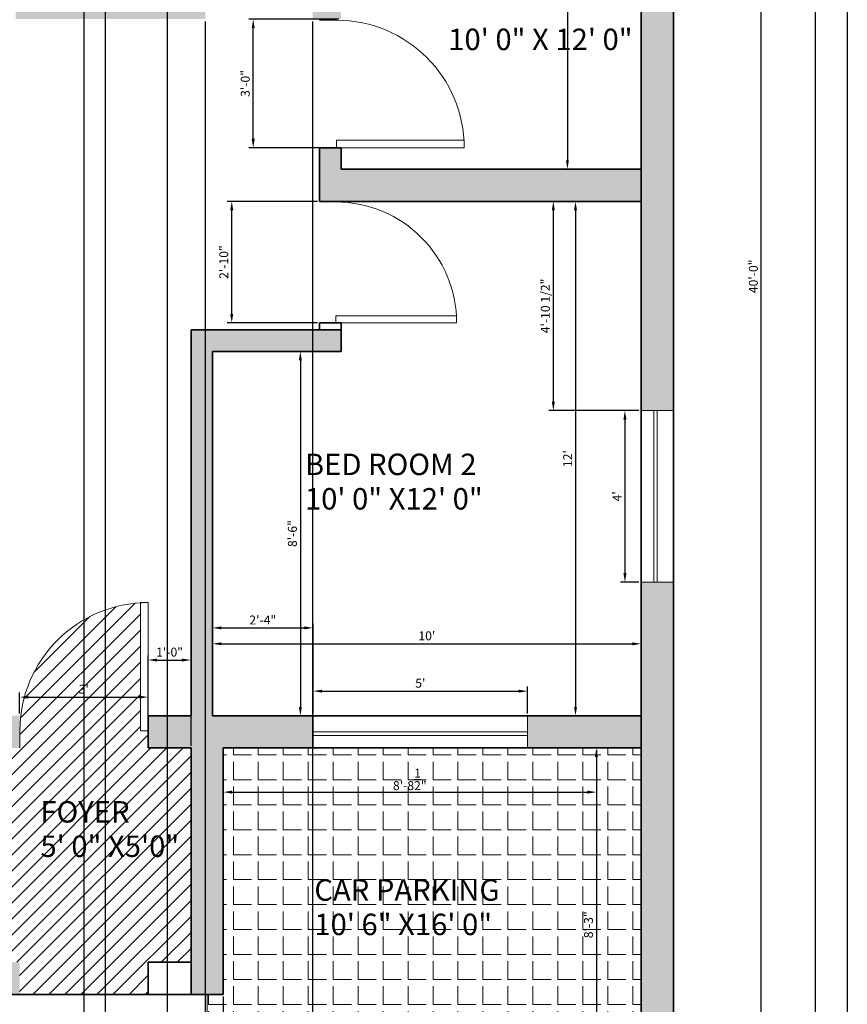
# Model space of a CAD drawing. Units: inches. Extents: x 2998 to 3448, y 1620 to 2377.
# Tile 3 of 5: x 3216 to 3448, y 1879 to 2155. Entities that reach past the tile are written whole.
import ezdxf

# ---------------------------------------------------------------- set-up
doc = ezdxf.new("R2010")
doc.units = ezdxf.units.IN
doc.layers.get('Defpoints').update_dxf_attribs({"color": 110})
for name, color, linetype, lineweight in [('A-ANNO-DIMS', 2, 'Continuous', 18), ('A-ANNO-TTLB', 7, 'Continuous', 25), ('A-AREA-IDEN', 130, 'Continuous', 18), ('A-DOOR', 3, 'Continuous', 18), ('A-FLOR-PATT', 18, 'Continuous', 13), ('A-GLAZ', 4, 'Continuous', 18), ('A-WALL-PATT', 18, 'Continuous', 13), ('C-PROP', 7, 'Continuous', 35), ('L-HRDS', 8, 'Continuous', 18), ('L-HRDS-PATT', 175, 'Continuous', 13), ('WALL', 7, 'Continuous', 35)]:
    doc.layers.add(name, color=color, linetype=linetype, lineweight=lineweight)
doc.styles.get("Standard").update_dxf_attribs({"font": 'arial.ttf'})
doc.dimstyles.new('Copy of ISO-25', dxfattribs={"dimtxt": 2.5, "dimasz": 2.5, "dimexe": 1.25, "dimexo": 0.625, "dimtad": 1, "dimdec": 1, "dimlunit": 4, "dimtxsty": 'Standard', "dimcen": 2.5, "dimadec": 0, "dimazin": 0, "dimtfac": 1, "dimtdec": 1, "dimtmove": 0, "dimatfit": 3, "dimfxl": 1, "dimarcsym": 0})

# ---------------------------------------------------------------- blocks, each defined once
blk = doc.blocks.new('*U3')
for p, q in [((-750, 0), (-750, -100)), ((0, 0), (0, -100))]:
    blk.add_line(p, q)
blk.add_lwpolyline([(0, 0), (0, 750), (-43.75, 750), (-43.75, 0)], close=True)
blk.add_arc((0, 0), 750, 90, 180)
blk = doc.blocks.new('*D4')
at = {"layer": 'A-ANNO-DIMS', "color": 0, "lineweight": -2, "transparency": 16777216}
for p, q in [((3389.49, 1950.77), (3376.33, 1950.77)), ((3377.58, 1948.27), (3377.58, 1854.27)), ((3389.49, 1851.77), (3376.33, 1851.77))]:
    blk.add_line(p, q, dxfattribs=at)
at = {"layer": 'A-ANNO-DIMS', "color": 0, "transparency": 16777216}
for points in [[(3377.16, 1948.27), (3378, 1948.27), (3377.58, 1950.77)], [(3377.16, 1854.27), (3378, 1854.27), (3377.58, 1851.77)]]:
    blk.add_solid(points, dxfattribs=at)
at = {"layer": 'Defpoints', "color": 0, "transparency": 16777216}
for p in [(3390.12, 1950.77), (3377.58, 1851.77), (3390.12, 1851.77)]:
    blk.add_point(p, dxfattribs=at)
at = {"layer": 'A-ANNO-DIMS', "color": 0, "transparency": 16777216, "insert": (3375.68, 1901.27), "char_height": 2.5, "attachment_point": 5, "rotation": 90}
blk.add_mtext('8\'-3"', dxfattribs=at)
blk = doc.blocks.new('*D13')
at = {"layer": 'A-ANNO-DIMS', "color": 0, "lineweight": -2, "transparency": 16777216}
for p, q in [((3389.49, 2256.77), (3368.21, 2256.77)), ((3369.46, 2254.27), (3369.46, 2115.27)), ((3389.49, 2112.77), (3368.21, 2112.77))]:
    blk.add_line(p, q, dxfattribs=at)
at = {"layer": 'A-ANNO-DIMS', "color": 0, "transparency": 16777216}
for points in [[(3369.04, 2254.27), (3369.87, 2254.27), (3369.46, 2256.77)], [(3369.04, 2115.27), (3369.87, 2115.27), (3369.46, 2112.77)]]:
    blk.add_solid(points, dxfattribs=at)
at = {"layer": 'Defpoints', "color": 0, "transparency": 16777216}
for p in [(3390.12, 2256.77), (3369.46, 2112.77), (3390.12, 2112.77)]:
    blk.add_point(p, dxfattribs=at)
at = {"layer": 'A-ANNO-DIMS', "color": 0, "transparency": 16777216, "insert": (3367.58, 2184.77), "char_height": 2.5, "attachment_point": 5, "rotation": 90}
blk.add_mtext("12'", dxfattribs=at)
blk = doc.blocks.new('*D14')
at = {"layer": 'A-ANNO-DIMS', "color": 0, "lineweight": -2, "transparency": 16777216}
for p, q in [((3270.12, 1960.4), (3270.12, 1981.17)), ((3272.62, 1979.92), (3387.62, 1979.92)), ((3390.12, 1960.4), (3390.12, 1981.17))]:
    blk.add_line(p, q, dxfattribs=at)
at = {"layer": 'A-ANNO-DIMS', "color": 0, "transparency": 16777216}
for points in [[(3272.62, 1980.33), (3272.62, 1979.5), (3270.12, 1979.92)], [(3387.62, 1980.33), (3387.62, 1979.5), (3390.12, 1979.92)]]:
    blk.add_solid(points, dxfattribs=at)
at = {"layer": 'Defpoints', "color": 0, "transparency": 16777216}
for p in [(3390.12, 1979.92), (3270.12, 1959.77), (3390.12, 1959.77)]:
    blk.add_point(p, dxfattribs=at)
at = {"layer": 'A-ANNO-DIMS', "color": 0, "transparency": 16777216, "insert": (3330.12, 1981.82), "char_height": 2.5, "attachment_point": 5}
blk.add_mtext("10'", dxfattribs=at)
blk = doc.blocks.new('*D15')
at = {"layer": 'A-ANNO-DIMS', "color": 0, "lineweight": -2, "transparency": 16777216}
for p, q in [((3389.49, 2103.77), (3370.48, 2103.77)), ((3371.73, 2101.27), (3371.73, 1962.27)), ((3389.49, 1959.77), (3370.48, 1959.77))]:
    blk.add_line(p, q, dxfattribs=at)
at = {"layer": 'A-ANNO-DIMS', "color": 0, "transparency": 16777216}
for points in [[(3371.31, 2101.27), (3372.14, 2101.27), (3371.73, 2103.77)], [(3371.31, 1962.27), (3372.14, 1962.27), (3371.73, 1959.77)]]:
    blk.add_solid(points, dxfattribs=at)
at = {"layer": 'Defpoints', "color": 0, "transparency": 16777216}
for p in [(3390.12, 2103.77), (3371.73, 1959.77), (3390.12, 1959.77)]:
    blk.add_point(p, dxfattribs=at)
at = {"layer": 'A-ANNO-DIMS', "color": 0, "transparency": 16777216, "insert": (3369.85, 2031.77), "char_height": 2.5, "attachment_point": 5, "rotation": 90}
blk.add_mtext("12'", dxfattribs=at)
blk = doc.blocks.new('*D16')
at = {"layer": 'A-ANNO-DIMS', "color": 0, "lineweight": -2, "transparency": 16777216}
for p, q in [((3273.12, 1950.15), (3273.12, 1937.14)), ((3377.58, 1950.15), (3377.58, 1937.14)), ((3275.62, 1938.39), (3375.08, 1938.39))]:
    blk.add_line(p, q, dxfattribs=at)
at = {"layer": 'A-ANNO-DIMS', "color": 0, "transparency": 16777216}
for points in [[(3275.62, 1938.81), (3275.62, 1937.97), (3273.12, 1938.39)], [(3375.08, 1938.81), (3375.08, 1937.97), (3377.58, 1938.39)]]:
    blk.add_solid(points, dxfattribs=at)
at = {"layer": 'Defpoints', "color": 0, "transparency": 16777216}
for p in [(3273.12, 1950.77), (3377.58, 1950.77), (3377.58, 1938.39)]:
    blk.add_point(p, dxfattribs=at)
at = {"layer": 'A-ANNO-DIMS', "color": 0, "transparency": 16777216, "insert": (3325.35, 1941.96), "char_height": 2.5, "attachment_point": 5}
blk.add_mtext('8\'-8{\\H1x;\\S1/2;}"', dxfattribs=at)
blk = doc.blocks.new('*D20')
at = {"layer": 'A-ANNO-DIMS', "color": 0, "lineweight": -2, "transparency": 16777216}
for p, q in [((3216.12, 1960.4), (3216.12, 1966.24)), ((3252.12, 1960.4), (3252.12, 1966.24)), ((3218.62, 1964.99), (3249.62, 1964.99))]:
    blk.add_line(p, q, dxfattribs=at)
at = {"layer": 'A-ANNO-DIMS', "color": 0, "transparency": 16777216}
for points in [[(3218.62, 1965.4), (3218.62, 1964.57), (3216.12, 1964.99)], [(3249.62, 1965.4), (3249.62, 1964.57), (3252.12, 1964.99)]]:
    blk.add_solid(points, dxfattribs=at)
at = {"layer": 'Defpoints', "color": 0, "transparency": 16777216}
for p in [(3252.12, 1964.99), (3216.12, 1959.77), (3252.12, 1959.77)]:
    blk.add_point(p, dxfattribs=at)
at = {"layer": 'A-ANNO-DIMS', "color": 0, "transparency": 16777216, "insert": (3234.12, 1966.89), "char_height": 2.5, "attachment_point": 5}
blk.add_mtext("3'", dxfattribs=at)
blk = doc.blocks.new('*D21')
at = {"layer": 'A-ANNO-DIMS', "color": 0, "lineweight": -2, "transparency": 16777216}
for p, q in [((3298.3, 1960.4), (3298.3, 1967.92)), ((3358.3, 1960.4), (3358.3, 1967.92)), ((3300.8, 1966.67), (3355.8, 1966.67))]:
    blk.add_line(p, q, dxfattribs=at)
at = {"layer": 'A-ANNO-DIMS', "color": 0, "transparency": 16777216}
for points in [[(3300.8, 1967.08), (3300.8, 1966.25), (3298.3, 1966.67)], [(3355.8, 1967.08), (3355.8, 1966.25), (3358.3, 1966.67)]]:
    blk.add_solid(points, dxfattribs=at)
at = {"layer": 'Defpoints', "color": 0, "transparency": 16777216}
for p in [(3358.3, 1966.67), (3298.3, 1959.77), (3358.3, 1959.77)]:
    blk.add_point(p, dxfattribs=at)
at = {"layer": 'A-ANNO-DIMS', "color": 0, "transparency": 16777216, "insert": (3328.3, 1968.56), "char_height": 2.5, "attachment_point": 5}
blk.add_mtext("5'", dxfattribs=at)
blk = doc.blocks.new('*D22')
at = {"layer": 'A-ANNO-DIMS', "color": 0, "lineweight": -2, "transparency": 16777216}
for p, q in [((3389.49, 2045.2), (3384.3, 2045.2)), ((3385.55, 2042.7), (3385.55, 1999.7)), ((3389.49, 1997.2), (3384.3, 1997.2))]:
    blk.add_line(p, q, dxfattribs=at)
at = {"layer": 'A-ANNO-DIMS', "color": 0, "transparency": 16777216}
for points in [[(3385.13, 2042.7), (3385.97, 2042.7), (3385.55, 2045.2)], [(3385.13, 1999.7), (3385.97, 1999.7), (3385.55, 1997.2)]]:
    blk.add_solid(points, dxfattribs=at)
at = {"layer": 'Defpoints', "color": 0, "transparency": 16777216}
for p in [(3390.12, 2045.2), (3385.55, 1997.2), (3390.12, 1997.2)]:
    blk.add_point(p, dxfattribs=at)
at = {"layer": 'A-ANNO-DIMS', "color": 0, "transparency": 16777216, "insert": (3383.68, 2021.2), "char_height": 2.5, "attachment_point": 5, "rotation": 90}
blk.add_mtext("4'", dxfattribs=at)
blk = doc.blocks.new('WIN-48IN')
for p, q in [((0, 0), (0, 9)), ((0, 9), (48, 9)), ((48, 9), (48, 0)), ((0, 4.5), (48, 4.5)), ((0, 3.5), (48, 3.5))]:
    blk.add_line(p, q)
blk = doc.blocks.new('WIN-60IN')
for p, q in [((0, 0), (0, 9)), ((60, 9), (60, 0)), ((0, 4.5), (60, 4.5)), ((0, 3.5), (60, 3.5))]:
    blk.add_line(p, q)
blk = doc.blocks.new('*D40')
at = {"layer": 'A-ANNO-DIMS', "color": 0, "lineweight": -2, "transparency": 16777216}
for p, q in [((3399.74, 2322.77), (3424.97, 2322.77)), ((3423.72, 1845.27), (3423.72, 2320.27)), ((3399.74, 1842.77), (3424.97, 1842.77))]:
    blk.add_line(p, q, dxfattribs=at)
at = {"layer": 'A-ANNO-DIMS', "color": 0, "transparency": 16777216}
for points in [[(3423.3, 2320.27), (3424.14, 2320.27), (3423.72, 2322.77)], [(3423.3, 1845.27), (3424.14, 1845.27), (3423.72, 1842.77)]]:
    blk.add_solid(points, dxfattribs=at)
at = {"layer": 'Defpoints', "color": 0}
for p in [(3399.12, 2322.77), (3423.72, 2322.77), (3399.12, 1842.77)]:
    blk.add_point(p, dxfattribs=at)
at = {"layer": 'A-ANNO-DIMS', "color": 0, "transparency": 16777216, "insert": (3421.82, 2082.77), "char_height": 2.5, "attachment_point": 5, "rotation": 90}
blk.add_mtext('40\'-0"', dxfattribs=at)
blk = doc.blocks.new('*D45')
at = {"layer": 'A-ANNO-DIMS', "color": 0, "lineweight": -2, "transparency": 16777216}
for p, q in [((3273.12, 1881.15), (3273.12, 1816.92)), ((3390.12, 1851.15), (3390.12, 1816.92)), ((3275.62, 1818.17), (3387.62, 1818.17))]:
    blk.add_line(p, q, dxfattribs=at)
at = {"layer": 'A-ANNO-DIMS', "color": 0, "transparency": 16777216}
for points in [[(3275.62, 1818.59), (3275.62, 1817.76), (3273.12, 1818.17)], [(3387.62, 1818.59), (3387.62, 1817.76), (3390.12, 1818.17)]]:
    blk.add_solid(points, dxfattribs=at)
at = {"layer": 'Defpoints', "color": 0}
for p in [(3273.12, 1881.77), (3390.12, 1851.77), (3390.12, 1818.17)]:
    blk.add_point(p, dxfattribs=at)
at = {"layer": 'A-ANNO-DIMS', "color": 0, "transparency": 16777216, "insert": (3331.62, 1820.07), "char_height": 2.5, "attachment_point": 5}
blk.add_mtext('9\'-9"', dxfattribs=at)
blk = doc.blocks.new('*D52')
at = {"layer": 'A-ANNO-DIMS', "color": 0, "lineweight": -2, "transparency": 16777216}
for p, q in [((3240.12, 2256.15), (3240.12, 1816.92)), ((3257.48, 2256.15), (3257.48, 1816.92)), ((3242.62, 1818.17), (3254.98, 1818.17))]:
    blk.add_line(p, q, dxfattribs=at)
at = {"layer": 'A-ANNO-DIMS', "color": 0, "transparency": 16777216}
for points in [[(3242.62, 1818.59), (3242.62, 1817.76), (3240.12, 1818.17)], [(3254.98, 1818.59), (3254.98, 1817.76), (3257.48, 1818.17)]]:
    blk.add_solid(points, dxfattribs=at)
at = {"layer": 'Defpoints', "color": 0}
for p in [(3240.12, 2256.77), (3257.48, 2256.77), (3257.48, 1818.17)]:
    blk.add_point(p, dxfattribs=at)
at = {"layer": 'A-ANNO-DIMS', "color": 0, "transparency": 16777216, "insert": (3248.8, 1820.09), "char_height": 2.5, "attachment_point": 5}
blk.add_mtext('1\'-5 1/2"', dxfattribs=at)
blk = doc.blocks.new('*D55')
at = {"layer": 'A-ANNO-DIMS', "color": 0, "lineweight": -2, "transparency": 16777216}
for p, q in [((3268.12, 2154.15), (3268.12, 1816.92)), ((3298.12, 2154.15), (3298.12, 1816.92)), ((3270.62, 1818.17), (3295.62, 1818.17))]:
    blk.add_line(p, q, dxfattribs=at)
at = {"layer": 'A-ANNO-DIMS', "color": 0, "transparency": 16777216}
for points in [[(3270.62, 1818.59), (3270.62, 1817.76), (3268.12, 1818.17)], [(3295.62, 1818.59), (3295.62, 1817.76), (3298.12, 1818.17)]]:
    blk.add_solid(points, dxfattribs=at)
at = {"layer": 'Defpoints', "color": 0}
for p in [(3268.12, 2154.77), (3298.12, 2154.77), (3298.12, 1818.17)]:
    blk.add_point(p, dxfattribs=at)
at = {"layer": 'A-ANNO-DIMS', "color": 0, "transparency": 16777216, "insert": (3283.12, 1820.07), "char_height": 2.5, "attachment_point": 5}
blk.add_mtext('2\'-6"', dxfattribs=at)
blk = doc.blocks.new('*D58')
at = {"layer": 'A-ANNO-DIMS', "color": 0, "lineweight": -2, "transparency": 16777216}
for p, q in [((3305.49, 2154.77), (3280.27, 2154.77)), ((3281.52, 2121.27), (3281.52, 2152.27)), ((3305.49, 2118.77), (3280.27, 2118.77))]:
    blk.add_line(p, q, dxfattribs=at)
at = {"layer": 'A-ANNO-DIMS', "color": 0, "transparency": 16777216}
for points in [[(3281.1, 2152.27), (3281.94, 2152.27), (3281.52, 2154.77)], [(3281.1, 2121.27), (3281.94, 2121.27), (3281.52, 2118.77)]]:
    blk.add_solid(points, dxfattribs=at)
at = {"layer": 'Defpoints', "color": 0}
for p in [(3281.52, 2154.77), (3306.12, 2154.77), (3306.12, 2118.77)]:
    blk.add_point(p, dxfattribs=at)
at = {"layer": 'A-ANNO-DIMS', "color": 0, "transparency": 16777216, "insert": (3279.62, 2136.77), "char_height": 2.5, "attachment_point": 5, "rotation": 90}
blk.add_mtext('3\'-0"', dxfattribs=at)
blk = doc.blocks.new('*D59')
at = {"layer": 'A-ANNO-DIMS', "color": 0, "lineweight": -2, "transparency": 16777216}
for p, q in [((3299.49, 2103.77), (3274.27, 2103.77)), ((3275.52, 2072.27), (3275.52, 2101.27)), ((3299.49, 2069.77), (3274.27, 2069.77))]:
    blk.add_line(p, q, dxfattribs=at)
at = {"layer": 'A-ANNO-DIMS', "color": 0, "transparency": 16777216}
for points in [[(3275.1, 2101.27), (3275.94, 2101.27), (3275.52, 2103.77)], [(3275.1, 2072.27), (3275.94, 2072.27), (3275.52, 2069.77)]]:
    blk.add_solid(points, dxfattribs=at)
at = {"layer": 'Defpoints', "color": 0}
for p in [(3275.52, 2103.77), (3300.12, 2103.77), (3300.12, 2069.77)]:
    blk.add_point(p, dxfattribs=at)
at = {"layer": 'A-ANNO-DIMS', "color": 0, "transparency": 16777216, "insert": (3273.62, 2086.77), "char_height": 2.5, "attachment_point": 5, "rotation": 90}
blk.add_mtext('2\'-10"', dxfattribs=at)
blk = doc.blocks.new('*D62')
at = {"layer": 'A-ANNO-DIMS', "color": 0, "lineweight": -2, "transparency": 16777216}
for p, q in [((3389.49, 2103.77), (3364.27, 2103.77)), ((3365.52, 2047.7), (3365.52, 2101.27)), ((3389.49, 2045.2), (3364.27, 2045.2))]:
    blk.add_line(p, q, dxfattribs=at)
at = {"layer": 'A-ANNO-DIMS', "color": 0, "transparency": 16777216}
for points in [[(3365.1, 2101.27), (3365.94, 2101.27), (3365.52, 2103.77)], [(3365.1, 2047.7), (3365.94, 2047.7), (3365.52, 2045.2)]]:
    blk.add_solid(points, dxfattribs=at)
at = {"layer": 'Defpoints', "color": 0}
for p in [(3365.52, 2103.77), (3390.12, 2103.77), (3390.12, 2045.2)]:
    blk.add_point(p, dxfattribs=at)
at = {"layer": 'A-ANNO-DIMS', "color": 0, "transparency": 16777216, "insert": (3363.6, 2074.49), "char_height": 2.5, "attachment_point": 5, "rotation": 90}
blk.add_mtext('4\'-10 1/2"', dxfattribs=at)
blk = doc.blocks.new('*D66')
at = {"layer": 'A-ANNO-DIMS', "color": 0, "lineweight": -2, "transparency": 16777216}
for p, q in [((3270.12, 1960.4), (3270.12, 1985.62)), ((3298.3, 1960.4), (3298.3, 1985.62)), ((3272.62, 1984.37), (3295.8, 1984.37))]:
    blk.add_line(p, q, dxfattribs=at)
at = {"layer": 'A-ANNO-DIMS', "color": 0, "transparency": 16777216}
for points in [[(3272.62, 1984.79), (3272.62, 1983.96), (3270.12, 1984.37)], [(3295.8, 1984.79), (3295.8, 1983.96), (3298.3, 1984.37)]]:
    blk.add_solid(points, dxfattribs=at)
at = {"layer": 'Defpoints', "color": 0}
for p in [(3298.3, 1984.37), (3270.12, 1959.77), (3298.3, 1959.77)]:
    blk.add_point(p, dxfattribs=at)
at = {"layer": 'A-ANNO-DIMS', "color": 0, "transparency": 16777216, "insert": (3284.21, 1986.25), "char_height": 2.5, "attachment_point": 5}
blk.add_mtext('2\'-4"', dxfattribs=at)
blk = doc.blocks.new('*D67')
at = {"layer": 'A-ANNO-DIMS', "color": 0, "lineweight": -2, "transparency": 16777216}
for p, q in [((3234.12, 2160.15), (3234.12, 1816.92)), ((3240.12, 2160.15), (3240.12, 1816.92)), ((3231.62, 1818.17), (3229.12, 1818.17)), ((3234.12, 1818.17), (3240.12, 1818.17)), ((3242.62, 1818.17), (3253.01, 1818.17))]:
    blk.add_line(p, q, dxfattribs=at)
at = {"layer": 'A-ANNO-DIMS', "color": 0, "transparency": 16777216}
for points in [[(3231.62, 1818.59), (3231.62, 1817.76), (3234.12, 1818.17)], [(3242.62, 1818.59), (3242.62, 1817.76), (3240.12, 1818.17)]]:
    blk.add_solid(points, dxfattribs=at)
at = {"layer": 'Defpoints', "color": 0}
for p in [(3234.12, 2160.77), (3240.12, 2160.77), (3240.12, 1818.17)]:
    blk.add_point(p, dxfattribs=at)
at = {"layer": 'A-ANNO-DIMS', "color": 0, "transparency": 16777216, "insert": (3249.07, 1820.07), "char_height": 2.5, "attachment_point": 5}
blk.add_mtext('0\'-6"', dxfattribs=at)
blk = doc.blocks.new('*D68')
at = {"layer": 'A-ANNO-DIMS', "color": 0, "lineweight": -2, "transparency": 16777216}
for p, q in [((3270.74, 2061.77), (3295.97, 2061.77)), ((3294.72, 2059.27), (3294.72, 1962.27)), ((3270.74, 1959.77), (3295.97, 1959.77))]:
    blk.add_line(p, q, dxfattribs=at)
at = {"layer": 'A-ANNO-DIMS', "color": 0, "transparency": 16777216}
for points in [[(3294.3, 2059.27), (3295.14, 2059.27), (3294.72, 2061.77)], [(3294.3, 1962.27), (3295.14, 1962.27), (3294.72, 1959.77)]]:
    blk.add_solid(points, dxfattribs=at)
at = {"layer": 'Defpoints', "color": 0}
for p in [(3270.12, 2061.77), (3270.12, 1959.77), (3294.72, 1959.77)]:
    blk.add_point(p, dxfattribs=at)
at = {"layer": 'A-ANNO-DIMS', "color": 0, "transparency": 16777216, "insert": (3292.82, 2010.77), "char_height": 2.5, "attachment_point": 5, "rotation": 90}
blk.add_mtext('8\'-6"', dxfattribs=at)
blk = doc.blocks.new('*D73')
at = {"layer": 'A-ANNO-DIMS', "color": 0, "lineweight": -2, "transparency": 16777216}
for p, q in [((3252.12, 1951.4), (3252.12, 1976.62)), ((3264.12, 1951.4), (3264.12, 1976.62)), ((3254.62, 1975.37), (3261.62, 1975.37))]:
    blk.add_line(p, q, dxfattribs=at)
at = {"layer": 'A-ANNO-DIMS', "color": 0, "transparency": 16777216}
for points in [[(3254.62, 1975.79), (3254.62, 1974.96), (3252.12, 1975.37)], [(3261.62, 1975.79), (3261.62, 1974.96), (3264.12, 1975.37)]]:
    blk.add_solid(points, dxfattribs=at)
at = {"layer": 'Defpoints', "color": 0}
for p in [(3264.12, 1975.37), (3252.12, 1950.77), (3264.12, 1950.77)]:
    blk.add_point(p, dxfattribs=at)
at = {"layer": 'A-ANNO-DIMS', "color": 0, "transparency": 16777216, "insert": (3258.12, 1977.27), "char_height": 2.5, "attachment_point": 5}
blk.add_mtext('1\'-0"', dxfattribs=at)

msp = doc.modelspace()

# ---------------------------------------------------------------- hatches: boundary and pattern name
at = {"layer": 'A-FLOR-PATT'}
h = msp.add_hatch(dxfattribs=at)
h.set_pattern_fill('ANSI31', color=256)
h.paths.add_polyline_path([(3264.12, 1950.77), (3252.12, 1950.77), (3252.12, 1955.56), (3250.03, 1955.56), (3250.03, 1991.39, 0.39722), (3216.23, 1955.56), (3216.23, 1950.77), (3204.12, 1950.77), (3204.12, 1890.77), (3216.12, 1890.77), (3216.12, 1881.77), (3252.12, 1881.77), (3252.12, 1890.77), (3264.12, 1890.77)])
h.paths.add_polyline_path([(3343.37, 2313.77), (3048.12, 2313.77), (3048.12, 2265.77), (3059.91, 2265.77), (3059.91, 2296.51), (3061.95, 2296.51), (3061.95, 2296.45, -0.39722), (3094.97, 2261.45), (3095.91, 2265.77), (3343.37, 2265.77)])
h.paths.add_polyline_path([(3220.44, 1918.61), (3261.55, 1918.61), (3261.55, 1927.8), (3220.44, 1927.8)], flags=24)
h.paths.add_polyline_path([(3220.42, 1928.23), (3252.4, 1928.23), (3252.4, 1937.54), (3220.42, 1937.54)], flags=24)
h.paths.add_polyline_path([(3097.58, 2294.93), (3164.02, 2294.93), (3164.02, 2304.23), (3097.58, 2304.23)], flags=24)
at = {"layer": 'A-WALL-PATT'}
h = msp.add_hatch(color=256, dxfattribs=at)
h.dxf.hatch_style = 1
h.paths.add_polyline_path([(3399.12, 2322.77), (3039.12, 2322.77), (3039.12, 2132.57), (3048.12, 2132.57), (3048.12, 2154.77), (3048.12, 2313.77), (3390.12, 2313.77), (3390.12, 2227.86), (3399.12, 2227.86)])
h.paths.add_polyline_path([(3048.12, 2072.57), (3039.12, 2072.57), (3039.12, 2041.4), (3048.12, 2041.4)])
h.paths.add_polyline_path([(3399.12, 1997.2), (3390.12, 1997.2), (3390.12, 1851.77), (3274.41, 1851.77), (3274.41, 1842.77), (3399.12, 1842.77)])
h.paths.add_polyline_path([(3195.35, 1851.77), (3048.12, 1851.77), (3048.12, 1857.27), (3048.05, 1858.06), (3047.68, 1858.02), (3047.44, 1857.61), (3047.47, 1857.28), (3047.17, 1857.15), (3047.68, 1858.02), (3045.29, 1857.73), (3045.29, 1842.77), (3195.35, 1842.77)])
h.paths.add_polyline_path([(3399.12, 2167.86), (3390.12, 2167.86), (3390.12, 2112.77), (3390.12, 2103.77), (3390.12, 2045.2), (3399.12, 2045.2)])
h.paths.add_polyline_path([(3390.12, 2112.77), (3306.12, 2112.77), (3306.12, 2118.77), (3304.88, 2118.77), (3300.12, 2118.77), (3300.12, 2112.77), (3300.12, 2103.77), (3390.12, 2103.77)])
h.paths.add_polyline_path([(3257.48, 2265.77), (3214.13, 2265.77), (3214.13, 2256.77), (3257.48, 2256.77)], flags=17)
h.paths.add_polyline_path([(3325.36, 2265.77), (3281.48, 2265.77), (3281.48, 2256.77), (3300.12, 2256.77), (3325.36, 2256.77)], flags=17)
h.paths.add_polyline_path([(3390.12, 2265.77), (3373.36, 2265.77), (3373.36, 2256.77), (3390.12, 2256.77)], flags=17)
h.paths.add_polyline_path([(3190.13, 2265.77), (3155.91, 2265.77), (3155.91, 2256.77), (3190.13, 2256.77)], flags=17)
h.paths.add_polyline_path([(3306.12, 2256.77), (3300.12, 2256.77), (3300.12, 2160.77), (3298.12, 2160.77), (3298.12, 2154.77), (3300.12, 2154.77), (3306.12, 2154.77)], flags=17)
h.paths.add_polyline_path([(3240.12, 2256.77), (3234.12, 2256.77), (3234.12, 2160.77), (3215.01, 2160.77), (3215.01, 2154.77), (3268.12, 2154.77), (3268.12, 2158.71), (3268.12, 2160.77), (3240.12, 2160.77)], flags=17)
h.paths.add_polyline_path([(3174.12, 2256.77), (3168.12, 2256.77), (3168.12, 2160.77), (3138.26, 2160.77), (3138.26, 2154.77), (3174.12, 2154.77), (3185.01, 2154.77), (3185.01, 2158.71), (3185.01, 2160.77), (3174.12, 2160.77)], flags=17)
h.paths.add_polyline_path([(3090.26, 2160.77), (3048.12, 2160.77), (3048.12, 2154.77), (3090.26, 2154.77)], flags=17)
h.paths.add_polyline_path([(3072.12, 2058.77), (3048.12, 2058.77), (3048.12, 2049.77), (3072.12, 2049.77)])
h.paths.add_polyline_path([(3298.3, 1959.77), (3270.12, 1959.77), (3270.12, 2061.77), (3300.12, 2061.77), (3306.12, 2061.77), (3306.12, 2067.77), (3300.12, 2067.77), (3264.12, 2067.77), (3264.12, 2061.77), (3264.12, 1959.77), (3252.12, 1959.77), (3252.12, 1955.56), (3252.12, 1950.77), (3264.12, 1950.77), (3264.12, 1890.77), (3264.12, 1881.77), (3273.12, 1881.77), (3273.12, 1950.77), (3298.3, 1950.77)])
h.paths.add_polyline_path([(3390.12, 1959.77), (3358.3, 1959.77), (3358.3, 1950.77), (3390.12, 1950.77)], flags=17)
h.paths.add_polyline_path([(3216.12, 1959.77), (3154.02, 1959.77), (3154.02, 1950.77), (3216.12, 1950.77)])
h.paths.add_polyline_path([(3204.12, 1950.77), (3195.12, 1950.77), (3195.12, 1890.77), (3195.12, 1881.77), (3216.12, 1881.77), (3216.12, 1890.77), (3204.12, 1890.77)])
h.paths.add_polyline_path([(3094.02, 1959.77), (3048.12, 1959.77), (3048.12, 1950.77), (3094.02, 1950.77)])
h.paths.add_polyline_path([(3045.29, 1981.4), (3040.45, 1981.4), (3040.45, 1842.77), (3045.29, 1842.77), (3045.29, 1857.73)])
h.paths.add_polyline_path([(3059.91, 2261.45), (3059.91, 2265.77), (3048.12, 2265.77), (3048.12, 2256.77), (3059.91, 2256.77)], flags=17)
h.paths.add_polyline_path([(3107.91, 2265.77), (3095.91, 2265.77), (3095.91, 2256.77), (3107.91, 2256.77)], flags=17)
h.paths.add_polyline_path([(3274.41, 1851.77), (3264.12, 1851.77), (3264.12, 1846.71), (3264.12, 1842.77), (3274.41, 1842.77)])
h.paths.add_polyline_path([(3204.35, 1851.77), (3195.35, 1851.77), (3195.35, 1842.77), (3204.35, 1842.77), (3204.35, 1846.71)])
at = {"layer": 'L-HRDS-PATT'}
h = msp.add_hatch(dxfattribs=at)
h.set_pattern_fill('_USER', color=256, pattern_type=0)
h.set_pattern_definition([(0, (0, 0), (0, 1), [])])
h.paths.add_polyline_path([(3195.12, 1950.77), (3154.02, 1950.77), (3154.02, 1914.77), (3084.12, 1914.77), (3084.12, 1881.77), (3195.12, 1881.77), (3195.12, 1890.77)])
h.paths.add_polyline_path([(3107.62, 2003.86), (3160.38, 2003.86), (3160.38, 2013.05), (3107.62, 2013.05)], flags=9)
h.paths.add_polyline_path([(3107.6, 2013.48), (3161.48, 2013.48), (3161.48, 2022.79), (3107.6, 2022.79)], flags=9)
h.paths.add_polyline_path([(3162.21, 2109.19), (3212.64, 2109.19), (3212.64, 2118.38), (3162.21, 2118.38)], flags=9)
h.paths.add_polyline_path([(3162.19, 2118.81), (3194.63, 2118.81), (3194.63, 2128.12), (3162.19, 2128.12)], flags=9)
h.paths.add_polyline_path([(3334.58, 2144.47), (3389.67, 2144.47), (3389.67, 2153.66), (3334.58, 2153.66)], flags=9)
h.paths.add_polyline_path([(3334.56, 2154.09), (3390.29, 2154.09), (3390.29, 2163.4), (3334.56, 2163.4)], flags=9)
h.paths.add_polyline_path([(3245.01, 2216.14), (3288.45, 2216.14), (3288.45, 2225.33), (3245.01, 2225.33)], flags=9)
h.paths.add_polyline_path([(3244.99, 2225.76), (3277.44, 2225.76), (3277.44, 2235.07), (3244.99, 2235.07)], flags=9)
h.paths.add_polyline_path([(3181.61, 2212.67), (3207.44, 2212.67), (3207.44, 2221.86), (3181.61, 2221.86)], flags=9)
h.paths.add_polyline_path([(3181.59, 2222.28), (3214.03, 2222.28), (3214.03, 2231.6), (3181.59, 2231.6)], flags=9)
h.paths.add_polyline_path([(3075.92, 2206.31), (3126.35, 2206.31), (3126.35, 2215.5), (3075.92, 2215.5)], flags=9)
h.paths.add_polyline_path([(3075.9, 2215.93), (3115.79, 2215.93), (3115.79, 2225.24), (3075.9, 2225.24)], flags=9)
h.paths.add_polyline_path([(3097.58, 2294.93), (3164.02, 2294.93), (3164.02, 2304.23), (3097.58, 2304.23)], flags=9)
h = msp.add_hatch(dxfattribs=at)
h.set_pattern_fill('ANGLE', color=256)
h.set_pattern_definition([(0, (0, 0), (0, 6.985), [5.08, -1.905]), (90, (0, 0), (-6.985, 4e-16), [5.08, -1.905])])
h.paths.add_polyline_path([(3390.12, 1950.77), (3358.3, 1950.77), (3273.12, 1950.77), (3273.12, 1881.77), (3268.62, 1881.77), (3268.62, 1851.77), (3390.12, 1851.77)])
h.paths.add_polyline_path([(3334.58, 2144.47), (3389.67, 2144.47), (3389.67, 2153.66), (3334.58, 2153.66)], flags=9)
h.paths.add_polyline_path([(3334.56, 2154.09), (3390.29, 2154.09), (3390.29, 2163.4), (3334.56, 2163.4)], flags=9)
h.paths.add_polyline_path([(3220.44, 1918.61), (3261.55, 1918.61), (3261.55, 1927.8), (3220.44, 1927.8)], flags=9)
h.paths.add_polyline_path([(3220.42, 1928.23), (3252.4, 1928.23), (3252.4, 1937.54), (3220.42, 1937.54)], flags=9)
h.paths.add_polyline_path([(3220.62, 1853.01), (3246.55, 1853.01), (3246.55, 1862.32), (3220.62, 1862.32)], flags=9)
h.paths.add_polyline_path([(3084.85, 1856.81), (3130.62, 1856.81), (3130.62, 1866), (3084.85, 1866)], flags=9)
h.paths.add_polyline_path([(3084.83, 1866.42), (3123.8, 1866.42), (3123.8, 1875.73), (3084.83, 1875.73)], flags=9)
h.paths.add_polyline_path([(3297.1, 1896.73), (3349.87, 1896.73), (3349.87, 1905.92), (3297.1, 1905.92)], flags=24)
h.paths.add_polyline_path([(3297.08, 1906.35), (3357.94, 1906.35), (3357.94, 1915.66), (3297.08, 1915.66)], flags=24)
h.paths.add_polyline_path([(3107.62, 2003.86), (3160.38, 2003.86), (3160.38, 2013.05), (3107.62, 2013.05)], flags=9)
h.paths.add_polyline_path([(3107.6, 2013.48), (3161.48, 2013.48), (3161.48, 2022.79), (3107.6, 2022.79)], flags=9)
h.paths.add_polyline_path([(3294.47, 2015.87), (3347.23, 2015.87), (3347.23, 2025.06), (3294.47, 2025.06)], flags=9)
h.paths.add_polyline_path([(3294.45, 2025.49), (3350.19, 2025.49), (3350.19, 2034.8), (3294.45, 2034.8)], flags=9)
h.paths.add_polyline_path([(3162.21, 2109.19), (3212.64, 2109.19), (3212.64, 2118.38), (3162.21, 2118.38)], flags=9)
h.paths.add_polyline_path([(3162.19, 2118.81), (3194.63, 2118.81), (3194.63, 2128.12), (3162.19, 2128.12)], flags=9)
h.paths.add_polyline_path([(3075.92, 2206.31), (3126.35, 2206.31), (3126.35, 2215.5), (3075.92, 2215.5)], flags=9)
h.paths.add_polyline_path([(3075.9, 2215.93), (3115.79, 2215.93), (3115.79, 2225.24), (3075.9, 2225.24)], flags=9)

# ---------------------------------------------------------------- linework, layer by layer
at = {"layer": 'A-ANNO-TTLB'}
for points in [[(2998.07, 2376.74), (3447.79, 2376.74), (3447.79, 1619.66), (2998.07, 1619.66)], [(3007.07, 2367.74), (3438.79, 2367.74), (3438.79, 1628.66), (3007.07, 1628.66)]]:
    msp.add_lwpolyline(points, close=True, dxfattribs=at)
at = {"layer": 'A-GLAZ'}
for q in [(3298.3, 1959.77), (3298.3, 1959.77), (3310.3, 1959.77)]:
    msp.add_line((3358.3, 1959.77), q, dxfattribs=at)
at = {"layer": 'C-PROP'}
for points in [[(3039.12, 2322.77), (3399.12, 2322.77), (3399.12, 1842.77), (3039.12, 1842.77)], [(3048.12, 2313.77), (3390.12, 2313.77), (3390.12, 1851.77), (3048.12, 1851.77)]]:
    msp.add_lwpolyline(points, close=True, dxfattribs=at)
at = {"layer": 'L-HRDS'}
msp.add_line((3268.62, 1881.77), (3268.62, 1851.77), dxfattribs=at)
at = {"layer": 'WALL'}
for p, q in [((3390.12, 2256.77), (3390.12, 2112.77)), ((3300.12, 2112.77), (3300.12, 2118.77)), ((3300.12, 2118.77), (3306.12, 2118.77)), ((3306.12, 2118.77), (3306.12, 2112.77)), ((3300.12, 2103.77), (3300.12, 2112.77)), ((3390.12, 2112.77), (3306.12, 2112.77)), ((3390.12, 2112.77), (3390.12, 2103.77)), ((3390.12, 2103.77), (3300.12, 2103.77)), ((3390.12, 2103.77), (3390.12, 1959.77)), ((3390.12, 2103.77), (3390.12, 2045.2)), ((3264.12, 1959.77), (3264.12, 2067.77)), ((3264.12, 2067.77), (3270.12, 2067.77)), ((3300.12, 2067.77), (3264.12, 2067.77)), ((3264.12, 2067.77), (3264.12, 2061.77)), ((3306.12, 2069.77), (3300.12, 2069.77)), ((3300.12, 2069.77), (3300.12, 2067.77)), ((3300.12, 2067.77), (3306.12, 2067.77)), ((3306.12, 2067.77), (3306.12, 2069.77)), ((3306.12, 2061.77), (3306.12, 2067.77)), ((3270.12, 2061.77), (3270.12, 1959.77)), ((3270.12, 2061.77), (3300.12, 2061.77)), ((3300.12, 2061.77), (3306.12, 2061.77)), ((3252.12, 1950.77), (3252.12, 1959.77)), ((3252.12, 1959.77), (3264.12, 1959.77)), ((3390.12, 1959.77), (3270.12, 1959.77)), ((3390.12, 1959.77), (3390.12, 1950.77)), ((3264.12, 1950.77), (3252.12, 1950.77)), ((3264.12, 1950.77), (3252.12, 1950.77)), ((3264.12, 1950.77), (3264.12, 1890.77)), ((3390.12, 1950.77), (3273.12, 1950.77)), ((3273.12, 1881.77), (3273.12, 1950.77)), ((3390.12, 1950.77), (3358.3, 1950.77)), ((3264.12, 1890.77), (3252.12, 1890.77)), ((3264.12, 1890.77), (3252.12, 1890.77)), ((3252.12, 1890.77), (3252.12, 1881.77)), ((3264.12, 1890.77), (3264.12, 1881.77)), ((3195.12, 1881.77), (3264.12, 1881.77)), ((3264.12, 1881.77), (3273.12, 1881.77))]:
    msp.add_line(p, q, dxfattribs=at)

# ---------------------------------------------------------------- block references
at = {"layer": 'A-DOOR', "rotation": 270}
for p, xscale, yscale, zscale in [((3304.88, 2118.77), 0.047591827255283, 0.047591827255283, 0.047591827255283), ((3304.63, 2069.77), 0.0451003427044547, 0.0451003427044547, 0.0451003427044547)]:
    msp.add_blockref('*U3', p, dxfattribs=dict(at, xscale=xscale, yscale=yscale, zscale=zscale))
at = {"layer": 'A-DOOR', "xscale": 0.0478583154260825, "yscale": 0.0478583154260825, "zscale": 0.0478583154260825}
msp.add_blockref('*U3', (3252.12, 1955.56), dxfattribs=at)
at = {"layer": 'A-GLAZ', "rotation": 270.0000000000008}
msp.add_blockref('WIN-48IN', (3390.12, 2045.2), dxfattribs=at)
at = {"layer": 'A-GLAZ'}
msp.add_blockref('WIN-60IN', (3298.3, 1950.77), dxfattribs=at)

# ---------------------------------------------------------------- texts
at = {"layer": 'A-AREA-IDEN'}
for s, p in [('10\' 0" X 12\' 0"', (3336.11, 2146.11)), ('BED ROOM 2', (3296, 2027.14)), ('10\' 0" X12\' 0"', (3296, 2017.5)), ('FOYER', (3221.98, 1929.88)), ('5\' 0" X5\'0"', (3221.98, 1920.25)), ('CAR PARKING', (3298.63, 1908)), ('10\' 6" X16\' 0"', (3298.63, 1898.37))]:
    msp.add_text(s, height=6, dxfattribs=at).set_placement(p)

# ---------------------------------------------------------------- dimensions: what is measured, and where the dimension line sits
at = {"layer": 'A-ANNO-DIMS'}
for base, p1, p2, angle, override, picture, middle in [((3423.72, 2322.77), (3399.12, 1842.77), (3399.12, 2322.77), 90, {"dimdec": 1, "dimlfac": 1, "dimrnd": 0, "dimzin": 1, "dimdsep": 46, "dimlunit": 4, "dimfrac": 2}, '*D40', (3421.82, 2082.77)), ((3369.46, 2112.77), (3390.12, 2256.77), (3390.12, 2112.77), 90, {"dimclrd": 0, "dimclre": 0, "dimclrt": 0}, '*D13', (3367.58, 2184.77)), ((3281.52, 2154.77), (3306.12, 2118.77), (3306.12, 2154.77), 90, {"dimdec": 1, "dimlfac": 1, "dimrnd": 0, "dimzin": 1, "dimdsep": 46, "dimlunit": 4, "dimfrac": 2}, '*D58', (3279.62, 2136.77)), ((3275.52, 2103.77), (3300.12, 2069.77), (3300.12, 2103.77), 90, {"dimdec": 1, "dimlfac": 1, "dimrnd": 0, "dimzin": 1, "dimdsep": 46, "dimlunit": 4, "dimfrac": 2}, '*D59', (3273.62, 2086.77)), ((3365.52, 2103.77), (3390.12, 2045.2), (3390.12, 2103.77), 90, {"dimdec": 1, "dimlfac": 1, "dimrnd": 0, "dimzin": 1, "dimdsep": 46, "dimlunit": 4, "dimfrac": 2}, '*D62', (3363.6, 2074.49)), ((3371.73, 1959.77), (3390.12, 2103.77), (3390.12, 1959.77), 90, {"dimclrd": 0, "dimclre": 0, "dimclrt": 0}, '*D15', (3369.85, 2031.77)), ((3294.72, 1959.77), (3270.12, 2061.77), (3270.12, 1959.77), 270, {"dimdec": 1, "dimlfac": 1, "dimrnd": 0, "dimzin": 1, "dimdsep": 46, "dimlunit": 4, "dimfrac": 2}, '*D68', (3292.82, 2010.77)), ((3385.55, 1997.2), (3390.12, 2045.2), (3390.12, 1997.2), 90, {"dimclrd": 0, "dimclre": 0, "dimclrt": 0}, '*D22', (3383.68, 2021.2)), ((3377.58, 1851.77), (3390.12, 1950.77), (3390.12, 1851.77), 90, {"dimclrd": 0, "dimclre": 0, "dimclrt": 0}, '*D4', (3375.68, 1901.27))]:
    dim = msp.add_linear_dim(base=base, p1=p1, p2=p2, angle=angle, dimstyle='Copy of ISO-25', override=override, dxfattribs=at)
    dim.commit()
    dim.dimension.update_dxf_attribs({"geometry": picture, "text_midpoint": middle})
for base, p1, p2, override, picture, middle in [((3257.48, 1818.17), (3240.12, 2256.77), (3257.48, 2256.77), {"dimdec": 1, "dimlfac": 1, "dimrnd": 0, "dimzin": 1, "dimdsep": 46, "dimlunit": 4, "dimfrac": 2}, '*D52', (3248.8, 1820.09)), ((3240.12, 1818.17), (3234.12, 2160.77), (3240.12, 2160.77), {"dimdec": 1, "dimlfac": 1, "dimrnd": 0, "dimzin": 1, "dimdsep": 46, "dimlunit": 4, "dimfrac": 2}, '*D67', (3249.07, 1820.07)), ((3298.12, 1818.17), (3268.12, 2154.77), (3298.12, 2154.77), {"dimdec": 1, "dimlfac": 1, "dimrnd": 0, "dimzin": 1, "dimdsep": 46, "dimlunit": 4, "dimfrac": 2}, '*D55', (3283.12, 1820.07)), ((3298.3, 1984.37), (3270.12, 1959.77), (3298.3, 1959.77), {"dimdec": 1, "dimlfac": 1, "dimrnd": 0, "dimzin": 1, "dimdsep": 46, "dimlunit": 4, "dimfrac": 2}, '*D66', (3284.21, 1986.25)), ((3390.12, 1979.92), (3270.12, 1959.77), (3390.12, 1959.77), {"dimclrd": 0, "dimclre": 0, "dimclrt": 0}, '*D14', (3330.12, 1981.82)), ((3264.12, 1975.37), (3252.12, 1950.77), (3264.12, 1950.77), {"dimdec": 1, "dimlfac": 1, "dimrnd": 0, "dimzin": 1, "dimdsep": 46, "dimlunit": 4, "dimfrac": 2}, '*D73', (3258.12, 1977.27)), ((3252.12, 1964.99), (3216.12, 1959.77), (3252.12, 1959.77), {"dimclrd": 0, "dimclre": 0, "dimclrt": 0}, '*D20', (3234.12, 1966.89)), ((3358.3, 1966.67), (3298.3, 1959.77), (3358.3, 1959.77), {"dimclrd": 0, "dimclre": 0, "dimclrt": 0}, '*D21', (3328.3, 1968.56)), ((3377.58, 1938.39), (3273.12, 1950.77), (3377.58, 1950.77), {"dimclrd": 0, "dimclre": 0, "dimclrt": 0}, '*D16', (3325.35, 1941.96)), ((3390.12, 1818.17), (3273.12, 1881.77), (3390.12, 1851.77), {"dimdec": 1, "dimlfac": 1, "dimrnd": 0, "dimzin": 1, "dimdsep": 46, "dimlunit": 4, "dimfrac": 2}, '*D45', (3331.62, 1820.07))]:
    dim = msp.add_linear_dim(base=base, p1=p1, p2=p2, dimstyle='Copy of ISO-25', override=override, dxfattribs=at)
    dim.commit()
    dim.dimension.update_dxf_attribs({"geometry": picture, "text_midpoint": middle})

doc.saveas('drawing.dxf')
